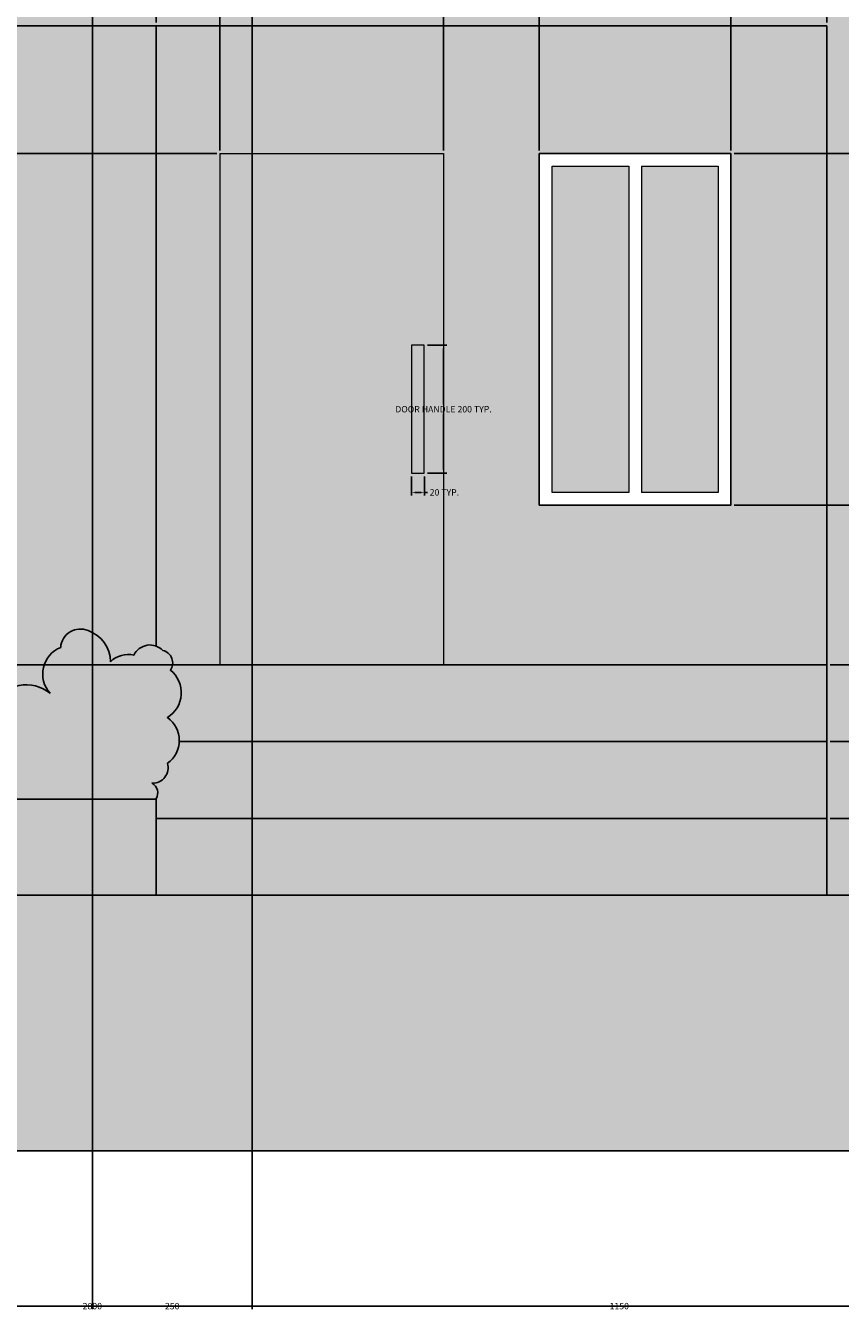
# Model space of a CAD drawing. Units: millimetres. Extents: x 2970 to 7764, y 2196 to 7505.
# Tile 4 of 13: x 5651 to 6927, y 2196 to 4206. Entities that reach past the tile are written whole.
import ezdxf

# ---------------------------------------------------------------- set-up
doc = ezdxf.new("R2010")
doc.units = ezdxf.units.MM
doc.header["$MEASUREMENT"] = 0
for name, color, linetype, lineweight in [('A-ANNO-DIMS', 2, 'Continuous', 18), ('A-DOOR', 3, 'Continuous', 18), ('A-ELEV', 7, 'Continuous', 25), ('A-ELEV-PATT', 8, 'Continuous', 13), ('A-GLAZ', 4, 'Continuous', 18)]:
    doc.layers.add(name, color=color, linetype=linetype, lineweight=lineweight)
doc.styles.get("Standard").update_dxf_attribs({"font": 'arial.ttf'})
doc.dimstyles.get("Standard").update_dxf_attribs({"dimtxt": 10, "dimasz": 5, "dimexe": 5, "dimexo": 5, "dimgap": 2, "dimtad": 0, "dimtih": 1, "dimtoh": 1, "dimdec": 0, "dimzin": 0, "dimdsep": 46, "dimtxsty": 'Standard', "dimcen": 2, "dimadec": 0, "dimazin": 0, "dimtfac": 1, "dimtdec": 0, "dimtofl": 0, "dimtmove": 0, "dimatfit": 3, "dimfxl": 1, "dimtolj": 1, "dimtzin": 0, "dimarcsym": 0})

# ---------------------------------------------------------------- blocks, each defined once
blk = doc.blocks.new('DOOR-HANDLE')
for p, q in [((20, 200), (0, 200)), ((0, 200), (0, 0)), ((20, 100), (20, 200)), ((20, 0), (20, 100)), ((0, 0), (20, 0))]:
    blk.add_line(p, q)
blk = doc.blocks.new('*D8')
at = {"layer": 'A-ANNO-DIMS', "color": 0, "lineweight": -2, "transparency": 16777216}
for p, q in [((6280.3, 3705.8), (6310.3, 3705.8)), ((6305.3, 3700.8), (6305.3, 3613)), ((6305.3, 3510.8), (6305.3, 3598.6)), ((6280.3, 3505.8), (6310.3, 3505.8))]:
    blk.add_line(p, q, dxfattribs=at)
at = {"layer": 'A-ANNO-DIMS', "color": 0, "transparency": 16777216}
for points in [[(6304.4, 3700.8), (6306.1, 3700.8), (6305.3, 3705.8)], [(6304.4, 3510.8), (6306.1, 3510.8), (6305.3, 3505.8)]]:
    blk.add_solid(points, dxfattribs=at)
at = {"layer": 'Defpoints', "color": 0, "transparency": 16777216}
for p in [(6275.3, 3705.8), (6305.3, 3705.8), (6275.3, 3505.8)]:
    blk.add_point(p, dxfattribs=at)
at = {"layer": 'A-ANNO-DIMS', "color": 0, "transparency": 16777216, "insert": (6305.3, 3605.8), "char_height": 10, "attachment_point": 5}
blk.add_mtext('\\A1;DOOR HANDLE 200 TYP.', dxfattribs=at)
blk = doc.blocks.new('*D9')
at = {"layer": 'A-ANNO-DIMS', "color": 0, "lineweight": -2, "transparency": 16777216}
for p, q in [((6255.3, 3500.8), (6255.3, 3470.8)), ((6275.3, 3500.8), (6275.3, 3470.8)), ((6260.3, 3475.8), (6270.3, 3475.8)), ((6275.3, 3475.8), (6280.3, 3475.8))]:
    blk.add_line(p, q, dxfattribs=at)
at = {"layer": 'A-ANNO-DIMS', "color": 0, "transparency": 16777216}
for points in [[(6260.3, 3476.6), (6260.3, 3475), (6255.3, 3475.8)], [(6270.3, 3476.6), (6270.3, 3475), (6275.3, 3475.8)]]:
    blk.add_solid(points, dxfattribs=at)
at = {"layer": 'Defpoints', "color": 0, "transparency": 16777216}
for p in [(6255.3, 3505.8), (6275.3, 3505.8), (6275.3, 3475.8)]:
    blk.add_point(p, dxfattribs=at)
at = {"layer": 'A-ANNO-DIMS', "color": 0, "transparency": 16777216, "insert": (6306.7, 3475.8), "char_height": 10, "attachment_point": 5}
blk.add_mtext('\\A1;20 TYP.', dxfattribs=at)
blk = doc.blocks.new('*D10')
at = {"layer": 'A-ANNO-DIMS', "color": 0, "lineweight": -2, "transparency": 16777216}
for p, q in [((3230.5, 2440.8), (3230.5, 2197.8)), ((7505.5, 2440.8), (7505.5, 2197.8)), ((3235.5, 2202.8), (5350.8, 2202.8)), ((7500.5, 2202.8), (5385.2, 2202.8))]:
    blk.add_line(p, q, dxfattribs=at)
at = {"layer": 'A-ANNO-DIMS', "color": 0, "transparency": 16777216}
for points in [[(3235.5, 2203.6), (3235.5, 2202), (3230.5, 2202.8)], [(7500.5, 2203.6), (7500.5, 2202), (7505.5, 2202.8)]]:
    blk.add_solid(points, dxfattribs=at)
at = {"layer": 'Defpoints', "color": 0, "transparency": 16777216}
for p in [(3230.5, 2445.8), (7505.5, 2445.8), (7505.5, 2202.8)]:
    blk.add_point(p, dxfattribs=at)
at = {"layer": 'A-ANNO-DIMS', "color": 0, "transparency": 16777216, "insert": (5368, 2202.8), "char_height": 10, "attachment_point": 5}
blk.add_mtext('\\A1;4275', dxfattribs=at)
blk = doc.blocks.new('*D37')
at = {"layer": 'A-ANNO-DIMS', "color": 0, "lineweight": -2, "transparency": 16777216}
for p, q in [((5855.3, 4210.8), (5855.3, 7503.8)), ((5860.3, 7498.8), (5892.7, 7498.8)), ((5950.3, 7498.8), (5917.8, 7498.8)), ((5955.3, 4010.8), (5955.3, 7503.8))]:
    blk.add_line(p, q, dxfattribs=at)
at = {"layer": 'A-ANNO-DIMS', "color": 0, "transparency": 16777216}
for points in [[(5860.3, 7499.6), (5860.3, 7498), (5855.3, 7498.8)], [(5950.3, 7499.6), (5950.3, 7498), (5955.3, 7498.8)]]:
    blk.add_solid(points, dxfattribs=at)
at = {"layer": 'Defpoints', "color": 0, "transparency": 16777216}
for p in [(5955.3, 7498.8), (5855.3, 4205.8), (5955.3, 4005.8)]:
    blk.add_point(p, dxfattribs=at)
at = {"layer": 'A-ANNO-DIMS', "color": 0, "transparency": 16777216, "insert": (5905.3, 7498.8), "char_height": 10, "attachment_point": 5}
blk.add_mtext('\\A1;100', dxfattribs=at)
blk = doc.blocks.new('*D38')
at = {"layer": 'A-ANNO-DIMS', "color": 0, "lineweight": -2, "transparency": 16777216}
for p, q in [((6755.3, 4010.8), (6755.3, 7503.8)), ((6760.3, 7498.8), (6808.1, 7498.8)), ((6900.5, 7498.8), (6852.7, 7498.8)), ((6905.5, 4210.8), (6905.5, 7503.8))]:
    blk.add_line(p, q, dxfattribs=at)
at = {"layer": 'A-ANNO-DIMS', "color": 0, "transparency": 16777216}
for points in [[(6760.3, 7499.6), (6760.3, 7498), (6755.3, 7498.8)], [(6900.5, 7499.6), (6900.5, 7498), (6905.5, 7498.8)]]:
    blk.add_solid(points, dxfattribs=at)
at = {"layer": 'Defpoints', "color": 0, "transparency": 16777216}
for p in [(6905.5, 7498.8), (6905.5, 4205.8), (6755.3, 4005.8)]:
    blk.add_point(p, dxfattribs=at)
at = {"layer": 'A-ANNO-DIMS', "color": 0, "transparency": 16777216, "insert": (6830.4, 7498.8), "char_height": 10, "attachment_point": 5}
blk.add_mtext('\\A1;150.23', dxfattribs=at)
blk = doc.blocks.new('*D39')
at = {"layer": 'A-ANNO-DIMS', "color": 0, "lineweight": -2, "transparency": 16777216}
for p, q in [((5955.3, 4010.8), (5955.3, 7503.8)), ((5960.3, 7498.8), (6117.2, 7498.8)), ((6300.3, 7498.8), (6143.3, 7498.8)), ((6305.3, 4010.8), (6305.3, 7503.8))]:
    blk.add_line(p, q, dxfattribs=at)
at = {"layer": 'A-ANNO-DIMS', "color": 0, "transparency": 16777216}
for points in [[(5960.3, 7499.6), (5960.3, 7498), (5955.3, 7498.8)], [(6300.3, 7499.6), (6300.3, 7498), (6305.3, 7498.8)]]:
    blk.add_solid(points, dxfattribs=at)
at = {"layer": 'Defpoints', "color": 0, "transparency": 16777216}
for p in [(6305.3, 7498.8), (5955.3, 4005.8), (6305.3, 4005.8)]:
    blk.add_point(p, dxfattribs=at)
at = {"layer": 'A-ANNO-DIMS', "color": 0, "transparency": 16777216, "insert": (6130.3, 7498.8), "char_height": 10, "attachment_point": 5}
blk.add_mtext('\\A1;350', dxfattribs=at)
blk = doc.blocks.new('*D40')
at = {"layer": 'A-ANNO-DIMS', "color": 0, "lineweight": -2, "transparency": 16777216}
for p, q in [((6305.3, 4010.8), (6305.3, 7503.8)), ((6310.3, 7498.8), (6367.7, 7498.8)), ((6450.3, 7498.8), (6392.8, 7498.8)), ((6455.3, 4010.8), (6455.3, 7503.8))]:
    blk.add_line(p, q, dxfattribs=at)
at = {"layer": 'A-ANNO-DIMS', "color": 0, "transparency": 16777216}
for points in [[(6310.3, 7499.6), (6310.3, 7498), (6305.3, 7498.8)], [(6450.3, 7499.6), (6450.3, 7498), (6455.3, 7498.8)]]:
    blk.add_solid(points, dxfattribs=at)
at = {"layer": 'Defpoints', "color": 0, "transparency": 16777216}
for p in [(6455.3, 7498.8), (6305.3, 4005.8), (6455.3, 4005.8)]:
    blk.add_point(p, dxfattribs=at)
at = {"layer": 'A-ANNO-DIMS', "color": 0, "transparency": 16777216, "insert": (6380.3, 7498.8), "char_height": 10, "attachment_point": 5}
blk.add_mtext('\\A1;150', dxfattribs=at)
blk = doc.blocks.new('*D41')
at = {"layer": 'A-ANNO-DIMS', "color": 0, "lineweight": -2, "transparency": 16777216}
for p, q in [((6455.3, 4010.8), (6455.3, 7503.8)), ((6460.3, 7498.8), (6592.2, 7498.8)), ((6750.3, 7498.8), (6618.3, 7498.8)), ((6755.3, 4010.8), (6755.3, 7503.8))]:
    blk.add_line(p, q, dxfattribs=at)
at = {"layer": 'A-ANNO-DIMS', "color": 0, "transparency": 16777216}
for points in [[(6460.3, 7499.6), (6460.3, 7498), (6455.3, 7498.8)], [(6750.3, 7499.6), (6750.3, 7498), (6755.3, 7498.8)]]:
    blk.add_solid(points, dxfattribs=at)
at = {"layer": 'Defpoints', "color": 0, "transparency": 16777216}
for p in [(6755.3, 7498.8), (6455.3, 4005.8), (6755.3, 4005.8)]:
    blk.add_point(p, dxfattribs=at)
at = {"layer": 'A-ANNO-DIMS', "color": 0, "transparency": 16777216, "insert": (6605.3, 7498.8), "char_height": 10, "attachment_point": 5}
blk.add_mtext('\\A1;300', dxfattribs=at)
blk = doc.blocks.new('*D43')
at = {"layer": 'A-ANNO-DIMS', "color": 0, "lineweight": -2, "transparency": 16777216}
for p, q in [((4355.5, 2840.8), (4355.5, 2197.8)), ((7155.5, 2840.8), (7155.5, 2197.8)), ((4360.5, 2202.8), (5738.5, 2202.8)), ((7150.5, 2202.8), (5772.5, 2202.8))]:
    blk.add_line(p, q, dxfattribs=at)
at = {"layer": 'A-ANNO-DIMS', "color": 0, "transparency": 16777216}
for points in [[(4360.5, 2203.6), (4360.5, 2202), (4355.5, 2202.8)], [(7150.5, 2203.6), (7150.5, 2202), (7155.5, 2202.8)]]:
    blk.add_solid(points, dxfattribs=at)
at = {"layer": 'Defpoints', "color": 0, "transparency": 16777216}
for p in [(4355.5, 2845.8), (7155.5, 2845.8), (7155.5, 2202.8)]:
    blk.add_point(p, dxfattribs=at)
at = {"layer": 'A-ANNO-DIMS', "color": 0, "transparency": 16777216, "insert": (5755.5, 2202.8), "char_height": 10, "attachment_point": 5}
blk.add_mtext('\\A1;2800', dxfattribs=at)
blk = doc.blocks.new('*D49')
at = {"layer": 'A-ANNO-DIMS', "color": 0, "lineweight": -2, "transparency": 16777216}
for p, q in [((5950.3, 4005.8), (2982.5, 4005.8)), ((2987.5, 4000.8), (2987.5, 3612.9)), ((2987.5, 3210.8), (2987.5, 3598.7)), ((5950.3, 3205.8), (2982.5, 3205.8))]:
    blk.add_line(p, q, dxfattribs=at)
at = {"layer": 'A-ANNO-DIMS', "color": 0, "transparency": 16777216}
for points in [[(2986.7, 4000.8), (2988.3, 4000.8), (2987.5, 4005.8)], [(2986.7, 3210.8), (2988.3, 3210.8), (2987.5, 3205.8)]]:
    blk.add_solid(points, dxfattribs=at)
at = {"layer": 'Defpoints', "color": 0, "transparency": 16777216}
for p in [(2987.5, 4005.8), (5955.3, 4005.8), (5955.3, 3205.8)]:
    blk.add_point(p, dxfattribs=at)
at = {"layer": 'A-ANNO-DIMS', "color": 0, "transparency": 16777216, "insert": (2987.5, 3605.8), "char_height": 10, "attachment_point": 5}
blk.add_mtext('\\A1;800', dxfattribs=at)
blk = doc.blocks.new('*D50')
at = {"layer": 'A-ANNO-DIMS', "color": 0, "lineweight": -2, "transparency": 16777216}
for p, q in [((6760.3, 3455.8), (7753.5, 3455.8)), ((7748.5, 3450.8), (7748.5, 3157.9)), ((7748.5, 2850.8), (7748.5, 3143.7)), ((7160.5, 2845.8), (7753.5, 2845.8))]:
    blk.add_line(p, q, dxfattribs=at)
at = {"layer": 'A-ANNO-DIMS', "color": 0, "transparency": 16777216}
for points in [[(7747.7, 3450.8), (7749.3, 3450.8), (7748.5, 3455.8)], [(7747.7, 2850.8), (7749.3, 2850.8), (7748.5, 2845.8)]]:
    blk.add_solid(points, dxfattribs=at)
at = {"layer": 'Defpoints', "color": 0, "transparency": 16777216}
for p in [(6755.3, 3455.8), (7748.5, 3455.8), (7155.5, 2845.8)]:
    blk.add_point(p, dxfattribs=at)
at = {"layer": 'A-ANNO-DIMS', "color": 0, "transparency": 16777216, "insert": (7748.5, 3150.8), "char_height": 10, "attachment_point": 5}
blk.add_mtext('\\A1;610', dxfattribs=at)
blk = doc.blocks.new('*D51')
at = {"layer": 'A-ANNO-DIMS', "color": 0, "lineweight": -2, "transparency": 16777216}
for p, q in [((6760.3, 4005.8), (7753.5, 4005.8)), ((7748.5, 4000.8), (7748.5, 3737.9)), ((7748.5, 3460.8), (7748.5, 3723.7)), ((6760.3, 3455.8), (7753.5, 3455.8))]:
    blk.add_line(p, q, dxfattribs=at)
at = {"layer": 'A-ANNO-DIMS', "color": 0, "transparency": 16777216}
for points in [[(7747.7, 4000.8), (7749.3, 4000.8), (7748.5, 4005.8)], [(7747.7, 3460.8), (7749.3, 3460.8), (7748.5, 3455.8)]]:
    blk.add_solid(points, dxfattribs=at)
at = {"layer": 'Defpoints', "color": 0, "transparency": 16777216}
for p in [(6755.3, 4005.8), (7748.5, 4005.8), (6755.3, 3455.8)]:
    blk.add_point(p, dxfattribs=at)
at = {"layer": 'A-ANNO-DIMS', "color": 0, "transparency": 16777216, "insert": (7748.5, 3730.8), "char_height": 10, "attachment_point": 5}
blk.add_mtext('\\A1;550', dxfattribs=at)
blk = doc.blocks.new('*D52')
at = {"layer": 'A-ANNO-DIMS', "color": 0, "lineweight": -2, "transparency": 16777216}
for p, q in [((7160.5, 4455.8), (7753.5, 4455.8)), ((7748.5, 4450.8), (7748.5, 4237.9)), ((7748.5, 4010.8), (7748.5, 4223.7)), ((6760.3, 4005.8), (7753.5, 4005.8))]:
    blk.add_line(p, q, dxfattribs=at)
at = {"layer": 'A-ANNO-DIMS', "color": 0, "transparency": 16777216}
for points in [[(7747.7, 4450.8), (7749.3, 4450.8), (7748.5, 4455.8)], [(7747.7, 4010.8), (7749.3, 4010.8), (7748.5, 4005.8)]]:
    blk.add_solid(points, dxfattribs=at)
at = {"layer": 'Defpoints', "color": 0, "transparency": 16777216}
for p in [(7155.5, 4455.8), (7748.5, 4455.8), (6755.3, 4005.8)]:
    blk.add_point(p, dxfattribs=at)
at = {"layer": 'A-ANNO-DIMS', "color": 0, "transparency": 16777216, "insert": (7748.5, 4230.8), "char_height": 10, "attachment_point": 5}
blk.add_mtext('\\A1;450', dxfattribs=at)
blk = doc.blocks.new('*D53')
at = {"layer": 'A-ANNO-DIMS', "color": 0, "lineweight": -2, "transparency": 16777216}
for p, q in [((6910.5, 2965.8), (7753.5, 2965.8)), ((7748.5, 2960.8), (7748.5, 2912.9)), ((7748.5, 2850.8), (7748.5, 2898.7)), ((6910.5, 2845.8), (7753.5, 2845.8))]:
    blk.add_line(p, q, dxfattribs=at)
at = {"layer": 'A-ANNO-DIMS', "color": 0, "transparency": 16777216}
for points in [[(7747.7, 2960.8), (7749.3, 2960.8), (7748.5, 2965.8)], [(7747.7, 2850.8), (7749.3, 2850.8), (7748.5, 2845.8)]]:
    blk.add_solid(points, dxfattribs=at)
at = {"layer": 'Defpoints', "color": 0, "transparency": 16777216}
for p in [(6905.5, 2965.8), (7748.5, 2965.8), (6905.5, 2845.8)]:
    blk.add_point(p, dxfattribs=at)
at = {"layer": 'A-ANNO-DIMS', "color": 0, "transparency": 16777216, "insert": (7748.5, 2905.8), "char_height": 10, "attachment_point": 5}
blk.add_mtext('\\A1;120', dxfattribs=at)
blk = doc.blocks.new('*D54')
at = {"layer": 'A-ANNO-DIMS', "color": 0, "lineweight": -2, "transparency": 16777216}
for p, q in [((6910.5, 3085.8), (7753.5, 3085.8)), ((7748.5, 3080.8), (7748.5, 3032.9)), ((7748.5, 2970.8), (7748.5, 3018.7)), ((6910.5, 2965.8), (7753.5, 2965.8))]:
    blk.add_line(p, q, dxfattribs=at)
at = {"layer": 'A-ANNO-DIMS', "color": 0, "transparency": 16777216}
for points in [[(7747.7, 3080.8), (7749.3, 3080.8), (7748.5, 3085.8)], [(7747.7, 2970.8), (7749.3, 2970.8), (7748.5, 2965.8)]]:
    blk.add_solid(points, dxfattribs=at)
at = {"layer": 'Defpoints', "color": 0, "transparency": 16777216}
for p in [(6905.5, 3085.8), (7748.5, 3085.8), (6905.5, 2965.8)]:
    blk.add_point(p, dxfattribs=at)
at = {"layer": 'A-ANNO-DIMS', "color": 0, "transparency": 16777216, "insert": (7748.5, 3025.8), "char_height": 10, "attachment_point": 5}
blk.add_mtext('\\A1;120', dxfattribs=at)
blk = doc.blocks.new('*D55')
at = {"layer": 'A-ANNO-DIMS', "color": 0, "lineweight": -2, "transparency": 16777216}
for p, q in [((6910.5, 3205.8), (7753.5, 3205.8)), ((7748.5, 3200.8), (7748.5, 3152.9)), ((7748.5, 3090.8), (7748.5, 3138.7)), ((6910.5, 3085.8), (7753.5, 3085.8))]:
    blk.add_line(p, q, dxfattribs=at)
at = {"layer": 'A-ANNO-DIMS', "color": 0, "transparency": 16777216}
for points in [[(7747.7, 3200.8), (7749.3, 3200.8), (7748.5, 3205.8)], [(7747.7, 3090.8), (7749.3, 3090.8), (7748.5, 3085.8)]]:
    blk.add_solid(points, dxfattribs=at)
at = {"layer": 'Defpoints', "color": 0, "transparency": 16777216}
for p in [(6905.5, 3205.8), (7748.5, 3205.8), (6905.5, 3085.8)]:
    blk.add_point(p, dxfattribs=at)
at = {"layer": 'A-ANNO-DIMS', "color": 0, "transparency": 16777216, "insert": (7748.5, 3145.8), "char_height": 10, "attachment_point": 5}
blk.add_mtext('\\A1;120', dxfattribs=at)
blk = doc.blocks.new('*D57')
at = {"layer": 'A-ANNO-DIMS', "color": 0, "lineweight": -2, "transparency": 16777216}
for p, q in [((5455.8, 5457.5), (5455.8, 2197.8)), ((5755.5, 5000.8), (5755.5, 2197.8)), ((5460.8, 2202.8), (5586.7, 2202.8)), ((5750.5, 2202.8), (5624.6, 2202.8))]:
    blk.add_line(p, q, dxfattribs=at)
at = {"layer": 'A-ANNO-DIMS', "color": 0, "transparency": 16777216}
for points in [[(5460.8, 2203.6), (5460.8, 2202), (5455.8, 2202.8)], [(5750.5, 2203.6), (5750.5, 2202), (5755.5, 2202.8)]]:
    blk.add_solid(points, dxfattribs=at)
at = {"layer": 'Defpoints', "color": 0, "transparency": 16777216}
for p in [(5455.8, 5462.5), (5755.5, 5005.8), (5755.5, 2202.8)]:
    blk.add_point(p, dxfattribs=at)
at = {"layer": 'A-ANNO-DIMS', "color": 0, "transparency": 16777216, "insert": (5605.7, 2202.8), "char_height": 10, "attachment_point": 5}
blk.add_mtext('\\A1;299.7', dxfattribs=at)
blk = doc.blocks.new('*D58')
at = {"layer": 'A-ANNO-DIMS', "color": 0, "lineweight": -2, "transparency": 16777216}
for p, q in [((6005.5, 5250.8), (6005.5, 2197.8)), ((5755.5, 5000.8), (5755.5, 2197.8)), ((5760.5, 2202.8), (5867.4, 2202.8)), ((6000.5, 2202.8), (5893.6, 2202.8))]:
    blk.add_line(p, q, dxfattribs=at)
at = {"layer": 'A-ANNO-DIMS', "color": 0, "transparency": 16777216}
for points in [[(5760.5, 2203.6), (5760.5, 2202), (5755.5, 2202.8)], [(6000.5, 2203.6), (6000.5, 2202), (6005.5, 2202.8)]]:
    blk.add_solid(points, dxfattribs=at)
at = {"layer": 'Defpoints', "color": 0, "transparency": 16777216}
for p in [(6005.5, 5255.8), (5755.5, 5005.8), (6005.5, 2202.8)]:
    blk.add_point(p, dxfattribs=at)
at = {"layer": 'A-ANNO-DIMS', "color": 0, "transparency": 16777216, "insert": (5880.5, 2202.8), "char_height": 10, "attachment_point": 5}
blk.add_mtext('\\A1;250', dxfattribs=at)
blk = doc.blocks.new('*D59')
at = {"layer": 'A-ANNO-DIMS', "color": 0, "lineweight": -2, "transparency": 16777216}
for p, q in [((6005.5, 5250.8), (6005.5, 2197.8)), ((7155.5, 5250.8), (7155.5, 2197.8)), ((6010.5, 2202.8), (6564.1, 2202.8)), ((7150.5, 2202.8), (6596.9, 2202.8))]:
    blk.add_line(p, q, dxfattribs=at)
at = {"layer": 'A-ANNO-DIMS', "color": 0, "transparency": 16777216}
for points in [[(6010.5, 2203.6), (6010.5, 2202), (6005.5, 2202.8)], [(7150.5, 2203.6), (7150.5, 2202), (7155.5, 2202.8)]]:
    blk.add_solid(points, dxfattribs=at)
at = {"layer": 'Defpoints', "color": 0, "transparency": 16777216}
for p in [(6005.5, 5255.8), (7155.5, 5255.8), (7155.5, 2202.8)]:
    blk.add_point(p, dxfattribs=at)
at = {"layer": 'A-ANNO-DIMS', "color": 0, "transparency": 16777216, "insert": (6580.5, 2202.8), "char_height": 10, "attachment_point": 5}
blk.add_mtext('\\A1;1150', dxfattribs=at)

msp = doc.modelspace()

# ---------------------------------------------------------------- hatches: boundary and pattern name
at = {"layer": 'A-ELEV-PATT'}
h = msp.add_hatch(color=256, dxfattribs=at)
h.dxf.hatch_style = 1
h.paths.add_polyline_path([(6405.5, 7255.789), (4305.5, 7255.789), (4305.5, 6505.789), (3730.5, 6505.789), (3730.5, 4205.789), (3730.5, 2945.789), (3730.5, 2895.789), (3830.5, 2895.789), (3830.5, 4205.789), (3830.5, 6405.789), (4405.5, 6405.789), (4405.5, 4205.789), (6905.5, 4205.789), (6905.5, 2945.789), (6905.5, 2845.789), (7155.5, 2845.789), (7155.5, 2945.789), (7155.5, 4205.789), (7155.5, 4455.789), (4555.5, 4455.789), (4555.5, 6505.789), (4555.5, 7005.789), (6155.5, 7005.789), (6155.5, 6755.789), (6405.5, 6755.789)])
h.paths.add_polyline_path([(7405.5, 6755.789), (6155.5, 6755.789), (5755.5, 6755.789), (5755.5, 5005.789), (7405.5, 5005.789)])
h.paths.add_polyline_path([(7155.5, 6505.789), (7155.5, 5255.789), (6005.5, 5255.789), (6005.5, 6505.789)], flags=16)
h.paths.add_polyline_path([(6105.5, 5520.789), (6105.5, 6055.789), (6455.5, 6055.789), (6455.5, 5520.789), (6655.5, 5520.789), (6655.5, 5605.789), (6655.5, 5955.789), (6955.5, 5955.789), (6955.5, 5605.789), (6955.5, 5520.789)], flags=0)
h.paths.add_polyline_path([(6425.5, 5755.789), (6425.5, 5655.789), (6425.5, 5555.789), (6405.5, 5555.789), (6405.5, 5755.789)], flags=0)
h.paths.add_polyline_path([(6955.5, 5505.789), (6955.5, 5405.789), (6655.5, 5405.789), (6655.5, 5505.789)], flags=0)
h = msp.add_hatch(color=256, dxfattribs=at)
h.set_gradient(color1=(199, 200, 202), color2=(147, 149, 152), name='INVSPHERICAL')
h.paths.add_polyline_path([(5254.666, 3214.122, -0.52056705), (5352.552, 3152.098, -0.4540886), (5432.911, 3123.272, -0.43983375), (5476.699, 3175.953, -0.52056705), (5498.186, 3233.206, -0.52056705), (5579.359, 3235.592, -0.52056705), (5588.909, 3164.025, -0.30236269), (5599.555, 3145.665, -0.44962196), (5689.182, 3161.64, -0.52056705), (5705.894, 3233.206, -0.52056705), (5748.868, 3259.448, -0.32013944), (5784.015, 3210.89, -0.25799727), (5820.491, 3221.279, -0.38376587), (5855.271, 3235.313), (5855.271, 4205.789), (5325.5, 4205.789), (5325.5, 3605.789), (4885.5, 3605.789), (4885.5, 4205.789), (4405.5, 4205.789), (4355.5, 4205.789), (4355.5, 3108.072, -0.29244748), (4395.384, 3104.368, -0.52056705), (4438.16, 3192.652, -0.52056705), (4519.333, 3216.508, -0.52056705), (4583.794, 3164.025, -0.37342356), (4571.284, 3103.834, -0.37512524), (4624.381, 3070.989, -0.49967099), (4754.056, 3098.592, -0.48686678), (4765.24, 3178.339, -0.52056705), (4827.314, 3199.809, -0.63134555), (4967.523, 3159.254, -0.19603193), (4962.635, 3135.756, -0.44420267), (5077.995, 3099.615, -0.52056705), (5156.781, 3159.254, -0.52056705)])
h.paths.add_polyline_path([(5450.5, 3618.289), (5475.5, 3718.289), (5475.5, 3893.289), (5450.5, 3993.289), (5600.5, 3993.289), (5575.5, 3893.289), (5575.5, 3718.289), (5600.5, 3618.289)], flags=16)
h.paths.add_polyline_path([(5490.5, 3733.289), (5490.5, 3878.289), (5560.5, 3878.289), (5560.5, 3733.289)], flags=0)
h.paths.add_polyline_path([(4760.5, 3618.289), (4610.5, 3618.289), (4635.5, 3718.289), (4635.5, 3893.289), (4610.5, 3993.289), (4760.5, 3993.289), (4735.5, 3893.289), (4735.5, 3718.289)], flags=16)
h.paths.add_polyline_path([(4720.5, 3733.289), (4650.5, 3733.289), (4650.5, 3878.289), (4720.5, 3878.289)], flags=0)
h = msp.add_hatch(color=256, dxfattribs=at)
h.set_gradient(color1=(147, 149, 152), color2=(199, 200, 202), name='SPHERICAL')
h.paths.add_polyline_path([(5855.271, 4205.789), (5855.271, 3235.313, -0.11402228), (5865.853, 3228.435, -0.38610396), (5881.03, 3205.789), (5955.271, 3205.789), (5955.271, 4005.789), (6305.271, 4005.789), (6305.271, 3205.789), (6905.5, 3205.789), (6905.5, 4205.789)])
h.paths.add_polyline_path([(6455.271, 4005.789), (6755.271, 4005.789), (6755.271, 3655.789), (6755.271, 3455.789), (6455.271, 3455.789), (6455.271, 3655.789)], flags=16)
h.paths.add_polyline_path([(6475.271, 3985.789), (6595.271, 3985.789), (6595.271, 3655.789), (6595.271, 3475.789), (6475.271, 3475.789), (6475.271, 3655.789)], flags=0)
h.paths.add_polyline_path([(6615.271, 3985.789), (6735.271, 3985.789), (6735.271, 3655.789), (6735.271, 3475.789), (6615.271, 3475.789), (6615.271, 3655.789)], flags=0)
h = msp.add_hatch(color=256, dxfattribs=at)
h.set_gradient(color1=(153, 76, 0), color2=(204, 102, 0))
h.paths.add_polyline_path([(5955.271, 3205.789), (6305.271, 3205.789), (6305.271, 4005.789), (5955.271, 4005.789)])
h.paths.add_polyline_path([(6255.271, 3705.789), (6275.271, 3705.789), (6275.271, 3605.789), (6275.271, 3505.789), (6255.271, 3505.789)], flags=16)
h = msp.add_hatch(color=256, dxfattribs=at)
h.set_gradient(color1=(122, 175, 223), color2=(173, 221, 247), name='SPHERICAL')
h.paths.add_polyline_path([(6615.271, 3655.789), (6615.271, 3475.789), (6735.271, 3475.789), (6735.271, 3655.789), (6735.271, 3985.789), (6615.271, 3985.789)])
h.paths.add_polyline_path([(6595.271, 3985.789), (6475.271, 3985.789), (6475.271, 3655.789), (6475.271, 3475.789), (6595.271, 3475.789), (6595.271, 3655.789)])
h = msp.add_hatch(color=256, dxfattribs=at)
h.set_gradient(color1=(248, 215, 49), color2=(247, 242, 129), name='SPHERICAL')
h.paths.add_polyline_path([(6275.271, 3605.789), (6275.271, 3705.789), (6255.271, 3705.789), (6255.271, 3505.789), (6275.271, 3505.789)])
h = msp.add_hatch(color=256, dxfattribs=at)
h.set_gradient(color1=(0, 255, 0), color2=(0, 153, 0), name='INVCURVED')
h.paths.add_polyline_path([(5156.781, 3159.254, 0.52056705), (5077.995, 3099.615, 0.44420267), (4962.635, 3135.756, 0.17969754), (4967.824, 3157.271, 0.6400553), (4827.314, 3199.809, 0.52056705), (4765.24, 3178.339, 0.48686678), (4754.056, 3098.592, -0.0165827), (4758.078, 3094.844, -0.02688608), (4754.056, 3098.592, 0.49967099), (4624.381, 3070.989, 0.37512524), (4571.284, 3103.834, 0.37342356), (4583.794, 3164.025, 0.52056705), (4519.333, 3216.508, 0.52056705), (4438.16, 3192.652, 0.52056705), (4395.384, 3104.368, 0.52056705), (4337.177, 3086.472, 0.52056705), (4340.162, 3038.75, 0.50842605), (4355.534, 2995.789), (5854.747, 2995.789, 0.43666624), (5849.141, 3020.892, 0.52056705), (5873.015, 3051.904, 0.52056705), (5873.015, 3123.471, 0.52056705), (5877.79, 3197.423, 0.52056705), (5865.853, 3228.435, 0.52056705), (5820.491, 3221.279, 0.25799727), (5784.015, 3210.89, 0.32013944), (5748.868, 3259.448, 0.52056705), (5705.894, 3233.206, 0.52056705), (5689.182, 3161.64, 0.44962196), (5599.555, 3145.665, 0.30236269), (5588.909, 3164.025, 0.52056705), (5579.359, 3235.592, 0.52056705), (5498.186, 3233.206, 0.52056705), (5476.699, 3175.953, 0.43983375), (5432.911, 3123.272, 0.4540886), (5352.552, 3152.098, 0.52056705), (5254.666, 3214.122, 0.52056705)])
h = msp.add_hatch(color=256, dxfattribs=at)
h.set_gradient(color1=(255, 255, 255), color2=(199, 200, 202), name='INVCYLINDER')
h.paths.add_polyline_path([(6905.5, 2965.789), (5855.271, 2965.789), (5855.271, 2845.789), (6905.5, 2845.789)])
h.paths.add_polyline_path([(5891.601, 3085.789), (6905.5, 3085.789), (6905.5, 3205.789), (5881.03, 3205.789, -0.11195993), (5877.79, 3197.423, -0.52056705), (5873.015, 3123.471, -0.25625024)])
h = msp.add_hatch(color=256, dxfattribs=at)
h.set_gradient(color1=(199, 200, 202), name='INVCYLINDER')
h.paths.add_polyline_path([(6905.5, 2965.789), (6905.5, 3085.789), (5891.601, 3085.789, -0.23320794), (5873.015, 3051.904, -0.52056705), (5849.141, 3020.892, -0.42041493), (5855.271, 2996.596), (5855.271, 2965.789)])
h = msp.add_hatch(color=256, dxfattribs=at)
h.set_gradient(color1=(76, 66, 38), color2=(0, 0, 0), name='INVSPHERICAL')
h.paths.add_polyline_path([(4355.5, 2995.789), (4355.5, 2895.789), (4355.5, 2845.789), (5855.271, 2845.789), (5855.271, 2995.789)])
h = msp.add_hatch(color=256, dxfattribs=at)
h.dxf.hatch_style = 1
h.paths.add_polyline_path([(7505.5, 2945.789), (7155.5, 2945.789), (7155.5, 2845.789), (6905.5, 2845.789), (4355.5, 2845.789), (4355.5, 2895.789), (3730.5, 2895.789), (3730.5, 2945.789), (3230.5, 2945.789), (3230.5, 2445.789), (7505.5, 2445.789)])

# ---------------------------------------------------------------- linework, layer by layer
at = {"layer": 'A-DOOR'}
for p, q in [((5955.271, 4005.789), (5955.271, 3205.789)), ((5955.271, 4005.789), (6305.271, 4005.789)), ((6305.271, 4005.789), (6305.271, 3205.789))]:
    msp.add_line(p, q, dxfattribs=at)
at = {"layer": 'A-ELEV'}
for p, q in [((4405.5, 4205.789), (6905.5, 4205.789)), ((5855.271, 4205.789), (5855.271, 3235.313)), ((6905.5, 4205.789), (6905.5, 2945.789)), ((6905.5, 3205.789), (5881.03, 3205.789)), ((6905.5, 2845.789), (6905.5, 3205.789)), ((6905.5, 3085.789), (5891.601, 3085.789)), ((4355.5, 2995.789), (5855.271, 2995.789)), ((5855.271, 2996.596), (5855.271, 2845.789)), ((6905.5, 2965.789), (5855.271, 2965.789)), ((6905.5, 2945.789), (6905.5, 2845.789)), ((6905.5, 2845.789), (4355.5, 2845.789)), ((6905.5, 2845.789), (7155.5, 2845.789)), ((7505.5, 2445.789), (3230.5, 2445.789))]:
    msp.add_line(p, q, dxfattribs=at)
for points in [[(6455.271, 3655.789), (6455.271, 4005.789), (6755.271, 4005.789), (6755.271, 3655.789)], [(6755.271, 3655.789), (6755.271, 3455.789), (6455.271, 3455.789), (6455.271, 3655.789)]]:
    msp.add_lwpolyline(points, dxfattribs=at)
for points in [[(5599.555, 3145.665, -0.44962196), (5689.182, 3161.64, -0.52056705), (5705.894, 3233.206, -0.52056705), (5748.868, 3259.448, -0.32013944), (5784.015, 3210.89)], [(5784.015, 3210.89, -0.25799727), (5820.491, 3221.279, -0.52056705), (5865.853, 3228.435, -0.52056705), (5877.79, 3197.423, -0.52056705), (5873.015, 3123.471, -0.52056705), (5873.015, 3051.904, -0.52056705), (5849.141, 3020.892, -0.42041493), (5855.271, 2996.596, -0.42041493)]]:
    msp.add_lwpolyline(points, format="xyb", dxfattribs=at)
at = {"layer": 'A-GLAZ'}
for p, q in [((6595.271, 3985.789), (6595.271, 3655.789)), ((6615.271, 3985.789), (6615.271, 3655.789)), ((6595.271, 3655.789), (6595.271, 3475.789)), ((6615.271, 3655.789), (6615.271, 3475.789))]:
    msp.add_line(p, q, dxfattribs=at)
for points in [[(6475.271, 3655.789), (6475.271, 3985.789), (6595.271, 3985.789)], [(6615.271, 3985.789), (6735.271, 3985.789), (6735.271, 3655.789)], [(6595.271, 3475.789), (6475.271, 3475.789), (6475.271, 3655.789)], [(6735.271, 3655.789), (6735.271, 3475.789), (6615.271, 3475.789)]]:
    msp.add_lwpolyline(points, dxfattribs=at)

# ---------------------------------------------------------------- block references
at = {"layer": 'A-DOOR'}
msp.add_blockref('DOOR-HANDLE', (6255.271, 3505.789), dxfattribs=at)

# ---------------------------------------------------------------- dimensions: what is measured, and where the dimension line sits
at = {"layer": 'A-ANNO-DIMS'}
for base, p1, p2, override, picture, middle in [((5955.271, 7498.789), (5855.271, 4205.789), (5955.271, 4005.789), {"dimdec": 0, "dimlfac": 1, "dimrnd": 0, "dimzin": 0, "dimdsep": 46, "dimlunit": 2}, '*D37', (5905.271, 7498.789)), ((6305.271, 7498.789), (5955.271, 4005.789), (6305.271, 4005.789), {"dimdec": 0, "dimlfac": 1, "dimrnd": 0, "dimzin": 0, "dimdsep": 46, "dimlunit": 2}, '*D39', (6130.271, 7498.789)), ((6455.271, 7498.789), (6305.271, 4005.789), (6455.271, 4005.789), {"dimdec": 0, "dimlfac": 1, "dimrnd": 0, "dimzin": 0, "dimdsep": 46, "dimlunit": 2}, '*D40', (6380.271, 7498.789)), ((6755.271, 7498.789), (6455.271, 4005.789), (6755.271, 4005.789), {"dimdec": 0, "dimlfac": 1, "dimrnd": 0, "dimzin": 0, "dimdsep": 46, "dimlunit": 2}, '*D41', (6605.271, 7498.789)), ((6905.5, 7498.789), (6755.271, 4005.789), (6905.5, 4205.789), {"dimdec": 2, "dimlfac": 1, "dimrnd": 0, "dimzin": 0, "dimdsep": 46, "dimlunit": 2}, '*D38', (6830.386, 7498.789)), ((5755.5, 2202.789), (5455.81, 5462.49), (5755.5, 5005.789), {"dimdec": 1, "dimlfac": 1, "dimrnd": 0, "dimzin": 0, "dimdsep": 46, "dimlunit": 2}, '*D57', (5605.655, 2202.789)), ((6005.5, 2202.789), (5755.5, 5005.789), (6005.5, 5255.789), {"dimdec": 0, "dimlfac": 1, "dimrnd": 0, "dimzin": 0, "dimdsep": 46, "dimlunit": 2}, '*D58', (5880.5, 2202.789)), ((7155.5, 2202.789), (6005.5, 5255.789), (7155.5, 5255.789), {"dimdec": 0, "dimlfac": 1, "dimrnd": 0, "dimzin": 0, "dimdsep": 46, "dimlunit": 2}, '*D59', (6580.5, 2202.789)), ((7155.5, 2202.789), (4355.5, 2845.789), (7155.5, 2845.789), {"dimdec": 0, "dimlfac": 1, "dimrnd": 0, "dimzin": 0, "dimdsep": 46, "dimlunit": 2}, '*D43', (5755.5, 2202.789)), ((7505.5, 2202.789), (3230.5, 2445.789), (7505.5, 2445.789), {"dimdec": 0, "dimlfac": 1, "dimrnd": 0, "dimzin": 0, "dimdsep": 46, "dimlunit": 2}, '*D10', (5368, 2202.789))]:
    dim = msp.add_linear_dim(base=base, p1=p1, p2=p2, dimstyle='Standard', override=override, dxfattribs=at)
    dim.commit()
    dim.dimension.update_dxf_attribs({"geometry": picture, "text_midpoint": middle})
for base, p1, p2, picture, middle in [((7748.5, 4455.789), (6755.271, 4005.789), (7155.5, 4455.789), '*D52', (7748.5, 4230.789)), ((2987.5, 4005.789), (5955.271, 3205.789), (5955.271, 4005.789), '*D49', (2987.5, 3605.789)), ((7748.5, 4005.789), (6755.271, 3455.789), (6755.271, 4005.789), '*D51', (7748.5, 3730.789)), ((7748.5, 3455.789), (7155.5, 2845.789), (6755.271, 3455.789), '*D50', (7748.5, 3150.789)), ((7748.5, 3205.789), (6905.5, 3085.789), (6905.5, 3205.789), '*D55', (7748.5, 3145.789)), ((7748.5, 3085.789), (6905.5, 2965.789), (6905.5, 3085.789), '*D54', (7748.5, 3025.789)), ((7748.5, 2965.789), (6905.5, 2845.789), (6905.5, 2965.789), '*D53', (7748.5, 2905.789))]:
    dim = msp.add_linear_dim(base=base, p1=p1, p2=p2, angle=90, dimstyle='Standard', override={"dimdec": 0, "dimlfac": 1, "dimrnd": 0, "dimzin": 0, "dimdsep": 46, "dimlunit": 2}, dxfattribs=at)
    dim.commit()
    dim.dimension.update_dxf_attribs({"geometry": picture, "text_midpoint": middle})
dim = msp.add_linear_dim(base=(6305.271, 3705.789), p1=(6275.271, 3505.789), p2=(6275.271, 3705.789), angle=90, text='DOOR HANDLE <> TYP.', dimstyle='Standard', override={"dimdec": 0, "dimlfac": 1, "dimrnd": 0, "dimzin": 0, "dimdsep": 46, "dimlunit": 2}, dxfattribs=at)
dim.commit()
dim.dimension.update_dxf_attribs({"geometry": '*D8', "text_midpoint": (6305.271, 3605.789)})
dim = msp.add_linear_dim(base=(6275.271, 3475.789), p1=(6255.271, 3505.789), p2=(6275.271, 3505.789), text='<> TYP.', dimstyle='Standard', override={"dimdec": 0, "dimlfac": 1, "dimrnd": 0, "dimzin": 0, "dimdsep": 46, "dimlunit": 2}, dxfattribs=at)
dim.commit()
dim.dimension.update_dxf_attribs({"geometry": '*D9', "text_midpoint": (6306.695, 3475.789)})

doc.saveas('drawing.dxf')
